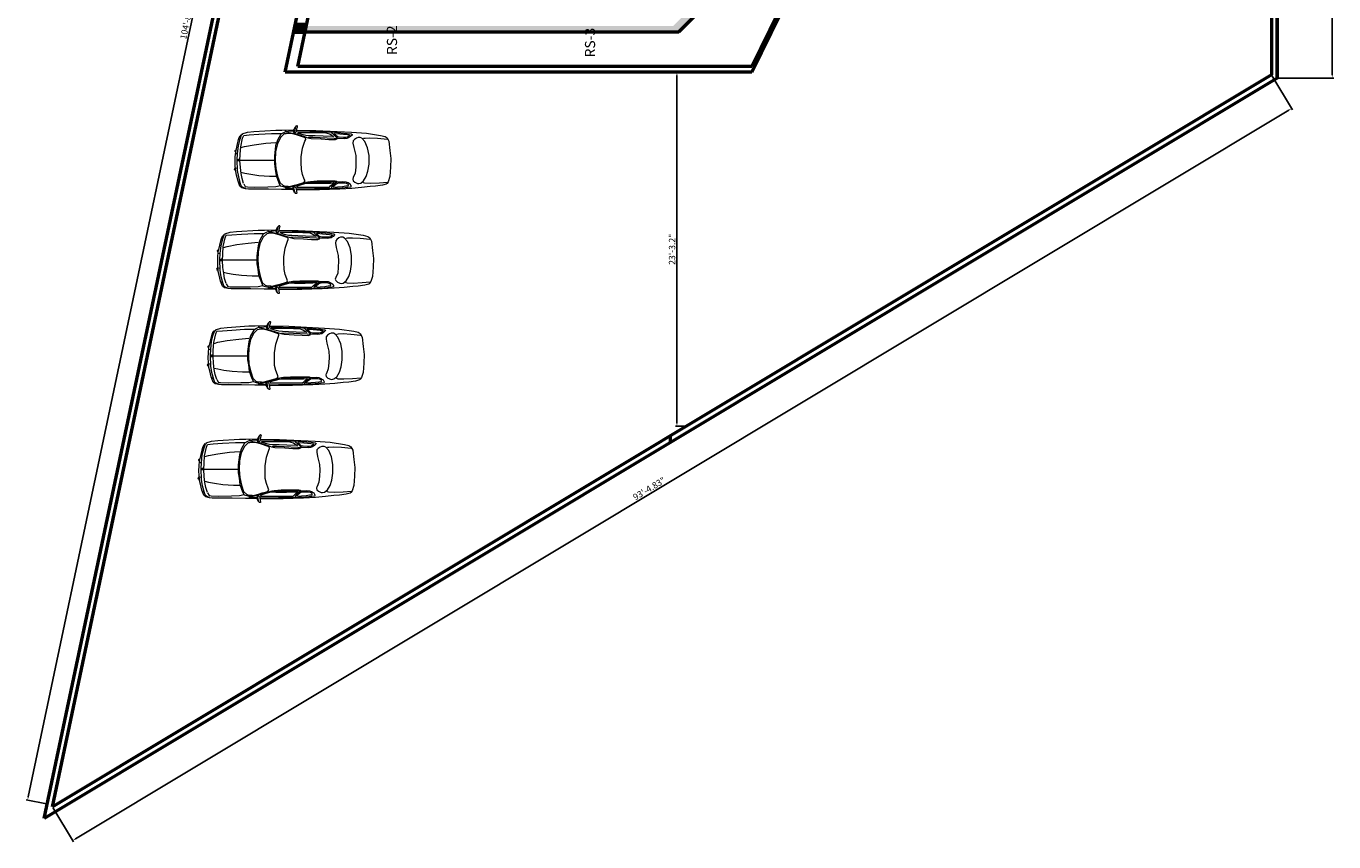
# Model space of a CAD drawing. Units: inches. Extents: x -2733 to 3435, y -338 to 1843.
# Tile 1 of 7: x -2733 to -1702, y -338 to 305. Entities that reach past the tile are written whole.
import ezdxf

# ---------------------------------------------------------------- set-up
doc = ezdxf.new("R2010")
doc.units = ezdxf.units.IN
doc.header["$PDMODE"] = 34
for name, color, linetype, lineweight in [('A-ANNO-DIMS', 2, 'Continuous', 18), ('A-ANNO-TEXT', 7, 'Continuous', 18), ('A-COLS', 1, 'Continuous', 35), ('A-WALL', 7, 'Continuous', 50), ('A-WALL-PATT', 8, 'Continuous', 13), ('C-PRKG', 8, 'Continuous', 18)]:
    doc.layers.add(name, color=color, linetype=linetype, lineweight=lineweight)
doc.styles.get("Standard").update_dxf_attribs({"font": 'arial.ttf'})
doc.styles.add('YQ_DIM', font='SUPEROS.SHX', dxfattribs={"width": 0.8, "bigfont": 'HZDX.SHX'})
doc.dimstyles.new('ISO-25', dxfattribs={"dimtxt": 5, "dimasz": 2.5, "dimexe": 1.25, "dimexo": 0.625, "dimtad": 1, "dimlunit": 3, "dimtxsty": 'Standard', "dimcen": 2.5, "dimadec": 0, "dimazin": 0, "dimtfac": 1, "dimtmove": 0, "dimatfit": 3, "dimfxl": 1, "dimarcsym": 0})

# ---------------------------------------------------------------- blocks, each defined once
blk = doc.blocks.new('A$C52303110')
for p, q in [((-1.969, 0.76), (-1.928, 0.839)), ((-1.928, 0.839), (-1.887, 0.875)), ((-1.928, 0.738), (-1.881, 0.868)), ((-1.881, 0.868), (-1.846, 0.889)), ((-1.863, 0.896), (-1.693, 0.951)), ((-1.852, 0.767), (-1.816, 0.853)), ((-1.816, 0.853), (-1.64, 0.868)), ((-1.693, 0.951), (-1.496, 0.973)), ((-1.64, 0.868), (-1.339, 0.889)), ((-1.496, 0.973), (-0.807, 1.016)), ((-1.339, 0.889), (-0.939, 0.911)), ((-0.939, 0.911), (-0.698, 0.911)), ((-0.807, 1.016), (-0.61, 1.016)), ((-0.647, 0.889), (-0.755, 0.7)), ((-0.698, 0.911), (-0.627, 0.911)), ((-0.539, 0.897), (-0.654, 0.79)), ((-0.56, 0.938), (-0.647, 0.889)), ((-0.61, 1.016), (-0.252, 1.027)), ((-0.499, 0.963), (-0.56, 0.938)), ((-0.479, 0.905), (-0.539, 0.897)), ((-0.517, 1.02), (-0.48, 0.966)), ((-0.404, 0.972), (-0.499, 0.963)), ((-0.48, 0.966), (-0.383, 0.946)), ((-0.371, 0.914), (-0.479, 0.905)), ((-0.256, 0.988), (-0.404, 0.972)), ((-0.383, 0.946), (-0.161, 0.897)), ((-0.263, 0.897), (-0.371, 0.914)), ((-0.115, 0.856), (-0.263, 0.897)), ((-0.237, 1.032), (-0.251, 1.001)), ((-0.251, 1.001), (-0.25, 0.98)), ((-0.25, 0.98), (-0.245, 0.957)), ((-0.245, 0.957), (-0.234, 0.947)), ((-0.198, 1.106), (-0.237, 1.032)), ((-0.234, 0.947), (-0.213, 0.938)), ((-0.206, 1.035), (-0.226, 0.944)), ((-0.213, 0.938), (-0.192, 0.936)), ((-0.185, 1.111), (-0.206, 1.035)), ((-0.184, 1.117), (-0.198, 1.106)), ((-0.192, 0.936), (-0.179, 0.942)), ((-0.168, 1.141), (-0.185, 1.111)), ((-0.179, 0.942), (-0.167, 0.957)), ((-0.162, 1.148), (-0.168, 1.141)), ((-0.167, 0.957), (-0.154, 0.98)), ((-0.142, 1.15), (-0.162, 1.148)), ((-0.161, 0.897), (0.098, 0.813)), ((-0.154, 0.98), (-0.148, 1.013)), ((-0.148, 1.013), (-0.144, 1.04)), ((-0.145, 0.991), (0.272, 0.981)), ((-0.144, 1.04), (-0.137, 1.07)), ((-0.144, 1.016), (0.455, 1.005)), ((-0.13, 1.15), (-0.142, 1.15)), ((-0.137, 1.07), (-0.123, 1.109)), ((-0.123, 1.145), (-0.13, 1.15)), ((-0.117, 1.134), (-0.123, 1.145)), ((-0.123, 1.109), (-0.117, 1.134)), ((-0.119, 0.926), (-0.109, 0.937)), ((0.017, 0.88), (-0.119, 0.926)), ((0.101, 0.782), (-0.115, 0.856)), ((-0.109, 0.937), (-0.091, 0.944)), ((-0.091, 0.944), (0.26, 0.948)), ((0.143, 0.85), (0.017, 0.88)), ((0.257, 0.843), (0.143, 0.85)), ((0.441, 0.835), (0.257, 0.843)), ((0.26, 0.948), (0.598, 0.941)), ((0.272, 0.981), (0.721, 0.966)), ((0.69, 0.824), (0.441, 0.835)), ((0.455, 1.005), (1.583, 0.951)), ((0.598, 0.941), (0.777, 0.937)), ((0.721, 0.966), (1.045, 0.951)), ((0.777, 0.937), (0.817, 0.926)), ((0.817, 0.926), (0.897, 0.896)), ((0.897, 0.896), (1.001, 0.832)), ((0.956, 0.951), (0.952, 0.971)), ((0.96, 0.926), (0.956, 0.951)), ((1.016, 0.877), (0.96, 0.926)), ((1.001, 0.832), (1.022, 0.813)), ((1.105, 0.798), (1.016, 0.877)), ((1.038, 0.912), (1.054, 0.916)), ((1.043, 0.899), (1.038, 0.912)), ((1.082, 0.858), (1.043, 0.899)), ((1.045, 0.951), (1.453, 0.917)), ((1.054, 0.916), (1.221, 0.903)), ((1.141, 0.807), (1.082, 0.858)), ((1.221, 0.903), (1.447, 0.882)), ((1.447, 0.882), (1.506, 0.871)), ((1.453, 0.917), (1.579, 0.897)), ((1.508, 0.83), (1.464, 0.796)), ((1.506, 0.871), (1.524, 0.86)), ((1.527, 0.847), (1.508, 0.83)), ((1.524, 0.86), (1.527, 0.847)), ((1.603, 0.862), (1.555, 0.818)), ((1.579, 0.897), (1.611, 0.882)), ((1.583, 0.951), (2.058, 0.918)), ((1.611, 0.882), (1.603, 0.862)), ((2.058, 0.918), (2.505, 0.852)), ((2.505, 0.852), (2.648, 0.819)), ((-2.069, 0.322), (-2.022, 0.537)), ((-2.022, 0.537), (-1.969, 0.76)), ((-2.01, 0.285), (-1.981, 0.523)), ((-1.981, 0.523), (-1.928, 0.738)), ((-1.975, 0.702), (-1.934, 0.738)), ((-1.928, 0.257), (-1.91, 0.494)), ((-1.91, 0.494), (-1.852, 0.767)), ((-1.904, 0.465), (-1.787, 0.501)), ((-1.787, 0.501), (-1.487, 0.559)), ((-1.487, 0.559), (-1.122, 0.602)), ((-1.122, 0.602), (-0.804, 0.631)), ((-0.809, 0.518), (-0.849, 0.206)), ((-0.755, 0.7), (-0.809, 0.518)), ((-0.755, 0.585), (-0.809, 0.329)), ((-0.654, 0.79), (-0.755, 0.585)), ((0, 0.173), (0.04, 0.445)), ((0.04, 0.445), (0.115, 0.667)), ((0.098, 0.813), (0.203, 0.778)), ((0.142, 0.757), (0.101, 0.782)), ((0.115, 0.667), (0.142, 0.724)), ((0.142, 0.724), (0.142, 0.757)), ((0.203, 0.778), (0.312, 0.754)), ((0.268, 0.783), (0.22, 0.783)), ((0.361, 0.788), (0.268, 0.783)), ((0.312, 0.754), (0.624, 0.739)), ((0.6, 0.778), (0.361, 0.788)), ((1.037, 0.759), (0.6, 0.778)), ((0.624, 0.739), (0.871, 0.724)), ((1.022, 0.813), (0.69, 0.824)), ((0.871, 0.724), (1.077, 0.719)), ((1.364, 0.748), (1.037, 0.759)), ((1.077, 0.719), (1.13, 0.739)), ((1.138, 0.763), (1.105, 0.798)), ((1.13, 0.739), (1.138, 0.763)), ((1.159, 0.801), (1.141, 0.807)), ((1.199, 0.794), (1.159, 0.801)), ((1.338, 0.788), (1.199, 0.794)), ((1.403, 0.79), (1.338, 0.788)), ((1.437, 0.759), (1.364, 0.748)), ((1.464, 0.796), (1.403, 0.79)), ((1.494, 0.773), (1.437, 0.759)), ((1.555, 0.818), (1.494, 0.773)), ((1.638, 0.675), (1.632, 0.604)), ((1.632, 0.604), (1.655, 0.471)), ((1.678, 0.724), (1.638, 0.675)), ((1.655, 0.471), (1.718, 0.217)), ((1.742, 0.767), (1.678, 0.724)), ((1.794, 0.788), (1.742, 0.767)), ((1.863, 0.788), (1.794, 0.788)), ((1.915, 0.76), (1.863, 0.788)), ((2.007, 0.661), (1.915, 0.76)), ((1.955, 0.738), (1.967, 0.76)), ((1.967, 0.76), (2.013, 0.767)), ((2.094, 0.457), (2.007, 0.661)), ((2.013, 0.767), (2.169, 0.774)), ((2.14, 0.217), (2.094, 0.457)), ((2.169, 0.774), (2.411, 0.76)), ((2.411, 0.76), (2.717, 0.731)), ((2.648, 0.819), (2.711, 0.776)), ((2.711, 0.776), (2.765, 0.666)), ((2.765, 0.666), (2.8, 0.371)), ((-2.087, 0.379), (-2.099, 0.364)), ((-2.099, 0.364), (-2.099, 0.35)), ((-2.099, 0.35), (-2.087, 0.343)), ((-2.064, 0.386), (-2.087, 0.379)), ((-2.087, 0.343), (-2.069, 0.336)), ((-2.087, 0.012), (-2.081, 0.17)), ((-2.081, -0.132), (-2.087, 0.012)), ((-2.081, 0.17), (-2.069, 0.322)), ((-2.057, 0.278), (-2.022, 0.285)), ((-2.022, 0.077), (-2.01, 0.285)), ((-2.01, -0.254), (-2.022, 0.077)), ((-1.981, 0.093), (-1.999, 0.079)), ((-1.999, 0.079), (-1.999, 0.064)), ((-1.999, 0.057), (-1.97, 0.057)), ((-1.963, 0.093), (-1.981, 0.093)), ((-1.97, 0.057), (-1.958, 0.057)), ((-1.958, 0.079), (-1.963, 0.093)), ((-1.958, 0.057), (-1.958, 0.079)), ((-1.934, 0.055), (-1.928, 0.257)), ((-1.922, -0.16), (-1.934, 0.055)), ((-1.926, 0.072), (-0.858, 0.072)), ((-0.849, 0.206), (-0.849, -0.049)), ((-0.809, 0.329), (-0.823, 0.058)), ((-0.823, 0.058), (-0.802, -0.19)), ((0, 0), (0, 0.173)), ((0.007, -0.23), (0, 0)), ((1.718, 0.217), (1.724, 0.033)), ((1.724, 0.033), (1.718, -0.15)), ((2.14, -0.058), (2.14, 0.217)), ((2.8, 0.371), (2.828, 0.12)), ((2.828, 0.12), (2.819, -0.153)), ((-2.11, -0.2), (-2.122, -0.221)), ((-2.122, -0.221), (-2.11, -0.236)), ((-2.093, -0.193), (-2.11, -0.2)), ((-2.11, -0.236), (-2.093, -0.25)), ((-2.069, -0.29), (-2.081, -0.132)), ((-2.04, -0.405), (-2.069, -0.29)), ((-2.064, -0.175), (-2.016, -0.182)), ((-1.993, -0.592), (-2.04, -0.405)), ((-1.975, -0.455), (-2.01, -0.254)), ((-1.898, -0.354), (-1.922, -0.16)), ((-1.903, -0.313), (-1.782, -0.341)), ((-1.869, -0.512), (-1.898, -0.354)), ((-1.782, -0.341), (-1.593, -0.376)), ((-1.593, -0.376), (-1.335, -0.411)), ((-1.335, -0.411), (-1.002, -0.432)), ((-0.849, -0.049), (-0.823, -0.214)), ((-0.823, -0.214), (-0.796, -0.412)), ((-0.802, -0.19), (-0.748, -0.436)), ((-0.796, -0.412), (-0.708, -0.642)), ((0.04, -0.387), (0.007, -0.23)), ((0.094, -0.527), (0.04, -0.387)), ((1.701, -0.34), (1.643, -0.481)), ((1.718, -0.15), (1.701, -0.34)), ((2.053, -0.446), (2.105, -0.277)), ((2.105, -0.277), (2.14, -0.058)), ((2.819, -0.153), (2.8, -0.448)), ((-1.934, -0.754), (-1.993, -0.592)), ((-1.916, -0.678), (-1.975, -0.455)), ((-1.975, -0.62), (-1.934, -0.642)), ((-1.872, -0.809), (-1.934, -0.754)), ((-1.881, -0.764), (-1.916, -0.678)), ((-1.816, -0.8), (-1.881, -0.764)), ((-1.755, -0.831), (-1.872, -0.809)), ((-1.822, -0.671), (-1.869, -0.512)), ((-1.816, -0.678), (-1.769, -0.764)), ((-1.752, -0.829), (-1.816, -0.8)), ((-1.769, -0.764), (-1.699, -0.771)), ((-1.699, -0.771), (-1.463, -0.778)), ((-1.463, -0.778), (-1.057, -0.771)), ((-1.057, -0.771), (-0.804, -0.764)), ((-1.002, -0.432), (-0.784, -0.432)), ((-0.804, -0.764), (-0.657, -0.735)), ((-0.748, -0.436), (-0.681, -0.634)), ((-0.708, -0.642), (-0.661, -0.741)), ((-0.681, -0.634), (-0.586, -0.724)), ((-0.661, -0.741), (-0.573, -0.766)), ((-0.586, -0.724), (-0.519, -0.749)), ((-0.573, -0.766), (-0.445, -0.799)), ((-0.519, -0.749), (-0.445, -0.749)), ((-0.503, -0.844), (-0.477, -0.811)), ((-0.477, -0.811), (-0.434, -0.788)), ((-0.445, -0.749), (-0.411, -0.749)), ((-0.445, -0.799), (-0.29, -0.823)), ((-0.434, -0.788), (-0.331, -0.774)), ((-0.398, -0.757), (-0.324, -0.749)), ((-0.331, -0.774), (-0.171, -0.732)), ((-0.324, -0.749), (-0.209, -0.716)), ((-0.267, -0.838), (-0.264, -0.809)), ((-0.264, -0.809), (-0.255, -0.789)), ((-0.255, -0.789), (-0.236, -0.778)), ((-0.236, -0.778), (-0.216, -0.773)), ((-0.232, -0.803), (-0.233, -0.779)), ((-0.221, -0.857), (-0.232, -0.803)), ((-0.216, -0.773), (-0.2, -0.775)), ((-0.209, -0.716), (-0.088, -0.683)), ((-0.2, -0.775), (-0.184, -0.792)), ((-0.184, -0.792), (-0.171, -0.809)), ((-0.171, -0.732), (-0.002, -0.68)), ((-0.171, -0.809), (-0.164, -0.829)), ((-0.132, -0.75), (-0.148, -0.778)), ((-0.148, -0.778), (-0.132, -0.783)), ((0.028, -0.704), (-0.132, -0.75)), ((-0.132, -0.783), (-0.067, -0.783)), ((-0.088, -0.683), (0.054, -0.642)), ((-0.067, -0.783), (0.147, -0.783)), ((-0.002, -0.68), (0.109, -0.643)), ((0.143, -0.671), (0.028, -0.704)), ((0.054, -0.642), (0.101, -0.617)), ((0.121, -0.585), (0.094, -0.527)), ((0.101, -0.617), (0.121, -0.585)), ((0.109, -0.643), (0.178, -0.62)), ((0.216, -0.662), (0.143, -0.671)), ((0.147, -0.783), (0.529, -0.783)), ((0.178, -0.62), (0.288, -0.601)), ((0.266, -0.629), (0.212, -0.624)), ((0.342, -0.666), (0.216, -0.662)), ((0.346, -0.634), (0.266, -0.629)), ((0.288, -0.601), (0.506, -0.587)), ((0.503, -0.671), (0.342, -0.666)), ((0.518, -0.634), (0.346, -0.634)), ((0.671, -0.666), (0.503, -0.671)), ((0.506, -0.587), (0.881, -0.587)), ((0.682, -0.629), (0.518, -0.634)), ((0.529, -0.783), (0.786, -0.783)), ((0.92, -0.662), (0.671, -0.666)), ((0.675, -0.83), (0.9, -0.825)), ((0.943, -0.624), (0.682, -0.629)), ((0.786, -0.783), (0.889, -0.783)), ((0.881, -0.587), (1.069, -0.587)), ((0.889, -0.783), (0.927, -0.746)), ((0.9, -0.825), (1.057, -0.816)), ((1.011, -0.652), (0.92, -0.662)), ((0.927, -0.746), (0.985, -0.69)), ((1.118, -0.615), (0.943, -0.624)), ((0.954, -0.788), (0.946, -0.82)), ((0.946, -0.82), (0.95, -0.839)), ((1, -0.722), (0.954, -0.788)), ((0.985, -0.69), (1.042, -0.657)), ((1.034, -0.741), (0.996, -0.783)), ((1.092, -0.648), (1, -0.722)), ((1.004, -0.783), (1.145, -0.774)), ((1.042, -0.657), (1.011, -0.652)), ((1.099, -0.69), (1.034, -0.741)), ((1.057, -0.816), (1.287, -0.802)), ((1.069, -0.587), (1.107, -0.592)), ((1.13, -0.629), (1.092, -0.648)), ((1.141, -0.662), (1.099, -0.69)), ((1.107, -0.592), (1.122, -0.606)), ((1.161, -0.62), (1.118, -0.615)), ((1.122, -0.606), (1.13, -0.629)), ((1.18, -0.657), (1.141, -0.662)), ((1.145, -0.774), (1.298, -0.76)), ((1.314, -0.615), (1.161, -0.62)), ((1.294, -0.652), (1.18, -0.657)), ((1.592, -0.82), (1.216, -0.842)), ((1.287, -0.802), (1.474, -0.783)), ((1.371, -0.652), (1.294, -0.652)), ((1.298, -0.76), (1.405, -0.746)), ((1.413, -0.62), (1.314, -0.615)), ((1.432, -0.666), (1.371, -0.652)), ((1.405, -0.746), (1.474, -0.741)), ((1.478, -0.648), (1.413, -0.62)), ((1.489, -0.704), (1.432, -0.666)), ((1.474, -0.741), (1.489, -0.727)), ((1.474, -0.783), (1.574, -0.769)), ((1.547, -0.69), (1.478, -0.648)), ((1.489, -0.727), (1.489, -0.704)), ((1.574, -0.732), (1.547, -0.69)), ((1.577, -0.76), (1.574, -0.732)), ((1.574, -0.769), (1.577, -0.76)), ((1.905, -0.798), (1.592, -0.82)), ((1.638, -0.481), (1.626, -0.531)), ((1.626, -0.531), (1.638, -0.58)), ((1.638, -0.58), (1.69, -0.629)), ((1.69, -0.629), (1.771, -0.664)), ((1.771, -0.664), (1.817, -0.671)), ((1.817, -0.671), (1.875, -0.657)), ((1.875, -0.657), (1.967, -0.587)), ((2.174, -0.766), (1.905, -0.798)), ((1.938, -0.615), (1.955, -0.636)), ((1.955, -0.636), (2.001, -0.65)), ((1.967, -0.587), (2.053, -0.446)), ((2.001, -0.65), (2.186, -0.657)), ((2.344, -0.754), (2.174, -0.766)), ((2.186, -0.657), (2.469, -0.643)), ((2.559, -0.722), (2.344, -0.754)), ((2.469, -0.643), (2.723, -0.622)), ((2.684, -0.689), (2.559, -0.722)), ((2.711, -0.667), (2.684, -0.689)), ((2.747, -0.612), (2.711, -0.667)), ((2.8, -0.448), (2.747, -0.612)), ((-1.666, -0.842), (-1.755, -0.831)), ((-1.55, -0.842), (-1.666, -0.842)), ((-1.039, -0.842), (-1.55, -0.842)), ((-0.619, -0.853), (-1.039, -0.842)), ((-0.279, -0.853), (-0.619, -0.853)), ((-0.254, -0.869), (-0.267, -0.838)), ((-0.233, -0.91), (-0.254, -0.869)), ((-0.217, -0.944), (-0.233, -0.91)), ((-0.205, -0.935), (-0.221, -0.857)), ((-0.2, -0.956), (-0.217, -0.944)), ((-0.196, -0.961), (-0.205, -0.935)), ((-0.192, -0.972), (-0.196, -0.961)), ((-0.178, -0.984), (-0.192, -0.972)), ((-0.166, -0.986), (-0.178, -0.984)), ((-0.152, -0.987), (-0.166, -0.986)), ((-0.164, -0.829), (-0.161, -0.849)), ((-0.161, -0.849), (-0.152, -0.906)), ((-0.155, -0.839), (0.124, -0.835)), ((-0.01, -0.864), (-0.153, -0.864)), ((-0.152, -0.906), (-0.143, -0.972)), ((-0.146, -0.982), (-0.152, -0.987)), ((-0.143, -0.972), (-0.146, -0.982)), ((0.572, -0.864), (-0.01, -0.864)), ((0.124, -0.835), (0.419, -0.83)), ((0.419, -0.83), (0.675, -0.83)), ((1.216, -0.842), (0.572, -0.864))]:
    blk.add_line(p, q)
blk = doc.blocks.new('*D5')
at = {"layer": 'A-ANNO-DIMS', "color": 0, "lineweight": -2, "transparency": 16777216}
for p, q in [((-2473, 922.1), (-2730.9, -302.7)), ((-2457.7, 921.4), (-2473.7, 924.8)), ((-2716.6, -308.3), (-2732.6, -304.9))]:
    blk.add_line(p, q, dxfattribs=at)
at = {"layer": 'A-ANNO-DIMS', "color": 0, "lineweight": 20, "transparency": 16777216}
for points in [[(-2473.4, 922.2), (-2472.6, 922), (-2472.5, 924.6)], [(-2731.3, -302.6), (-2730.5, -302.8), (-2731.4, -305.2)]]:
    blk.add_solid(points, dxfattribs=at)
at = {"layer": 'Defpoints', "color": 0, "lineweight": 20, "transparency": 16777216}
for p in [(-2457, 921.3), (-2731.4, -305.2), (-2715.9, -308.4)]:
    blk.add_point(p, dxfattribs=at)
at = {"layer": 'A-ANNO-DIMS', "color": 0, "transparency": 16777216, "insert": (-2605, 310.4), "char_height": 5, "attachment_point": 5, "rotation": 78.1108}
blk.add_mtext('104\'-8.67"', dxfattribs=at)
blk = doc.blocks.new('*D6')
at = {"layer": 'A-ANNO-DIMS', "color": 0, "lineweight": -2, "transparency": 16777216}
for p, q in [((-1745.9, 1560.1), (-1701.9, 1560.1)), ((-1703.2, 1557.6), (-1703.2, 266.6)), ((-1745.9, 264.1), (-1701.9, 264.1))]:
    blk.add_line(p, q, dxfattribs=at)
at = {"layer": 'A-ANNO-DIMS', "color": 0, "lineweight": 20, "transparency": 16777216}
for points in [[(-1703.6, 1557.6), (-1702.8, 1557.6), (-1703.2, 1560.1)], [(-1703.6, 266.6), (-1702.8, 266.6), (-1703.2, 264.1)]]:
    blk.add_solid(points, dxfattribs=at)
at = {"layer": 'Defpoints', "color": 0, "lineweight": 20, "transparency": 16777216}
for p in [(-1746.6, 1560.1), (-1746.6, 264.1), (-1703.2, 264.1)]:
    blk.add_point(p, dxfattribs=at)
at = {"layer": 'A-ANNO-DIMS', "color": 0, "transparency": 16777216, "insert": (-1706.4, 912.1), "char_height": 5, "attachment_point": 5, "rotation": 90}
blk.add_mtext("108'", dxfattribs=at)
blk = doc.blocks.new('*D7')
at = {"layer": 'A-ANNO-DIMS', "color": 0, "lineweight": -2, "transparency": 16777216}
for p, q in [((-1750.7, 266.1), (-1734.5, 239.1)), ((-1737.3, 238.9), (-2693.7, -335.8)), ((-2711.5, -311.1), (-2695.2, -338.2))]:
    blk.add_line(p, q, dxfattribs=at)
at = {"layer": 'A-ANNO-DIMS', "color": 0, "lineweight": 20, "transparency": 16777216}
for points in [[(-1737.5, 239.2), (-1737.1, 238.5), (-1735.1, 240.2)], [(-2694, -335.4), (-2693.5, -336.2), (-2695.9, -337.1)]]:
    blk.add_solid(points, dxfattribs=at)
at = {"layer": 'Defpoints', "color": 0, "lineweight": 20, "transparency": 16777216}
for p in [(-1751.1, 266.7), (-2711.8, -310.6), (-2695.9, -337.1)]:
    blk.add_point(p, dxfattribs=at)
at = {"layer": 'A-ANNO-DIMS', "color": 0, "transparency": 16777216, "insert": (-2241.2, -60.2), "char_height": 5, "attachment_point": 5, "rotation": 31}
blk.add_mtext('93\'-4.83"', dxfattribs=at)
blk = doc.blocks.new('*D19')
at = {"layer": 'A-ANNO-DIMS', "color": 0, "lineweight": -2, "transparency": 16777216}
for p, q in [((-2213.5, 268.7), (-2220.9, 268.7)), ((-2219.7, 266.2), (-2219.7, -8)), ((-2213, -10.5), (-2220.9, -10.5))]:
    blk.add_line(p, q, dxfattribs=at)
at = {"layer": 'A-ANNO-DIMS', "color": 0, "lineweight": 20, "transparency": 16777216}
for points in [[(-2220.1, 266.2), (-2219.3, 266.2), (-2219.7, 268.7)], [(-2220.1, -8), (-2219.3, -8), (-2219.7, -10.5)]]:
    blk.add_solid(points, dxfattribs=at)
at = {"layer": 'Defpoints', "color": 0, "lineweight": 20, "transparency": 16777216}
for p in [(-2212.9, 268.7), (-2219.7, -10.5), (-2212.4, -10.5)]:
    blk.add_point(p, dxfattribs=at)
at = {"layer": 'A-ANNO-DIMS', "color": 0, "transparency": 16777216, "insert": (-2222.9, 129.1), "char_height": 5, "attachment_point": 5, "rotation": 90}
blk.add_mtext('23\'-3.2"', dxfattribs=at)
blk = doc.blocks.new('*D22')
at = {"layer": 'A-ANNO-DIMS', "color": 0, "lineweight": -2, "transparency": 16777216}
blk.add_arc((-2457, 921.3), 20.3, 94.064, 251.0467, dxfattribs=at)
at = {"layer": 'A-ANNO-DIMS', "color": 0, "lineweight": 20, "transparency": 16777216}
for points in [[(-2458.5, 942), (-2458.5, 941.1), (-2456, 941.6)], [(-2463.5, 902.5), (-2463.7, 901.7), (-2461.2, 901.5)]]:
    blk.add_solid(points, dxfattribs=at)
at = {"layer": 'Defpoints', "color": 0, "lineweight": 20, "transparency": 16777216}
for p in [(-2423.6, 1560.1), (-2473.5, 933.2), (-2457, 921.3), (-2457, 921.3), (-2718.3, -319.8)]:
    blk.add_point(p, dxfattribs=at)
at = {"layer": 'A-ANNO-DIMS', "color": 0, "transparency": 16777216, "insert": (-2480.3, 924.3), "char_height": 5, "attachment_point": 5, "rotation": 82.5554}
blk.add_mtext('171°', dxfattribs=at)

msp = doc.modelspace()

# ---------------------------------------------------------------- hatches: boundary and pattern name
at = {"layer": 'A-COLS'}
h = msp.add_hatch(color=256, dxfattribs=at)
h.dxf.hatch_style = 1
h.paths.add_polyline_path([(-2512.158, 307.862), (-2521.158, 307.862), (-2521.158, 298.862), (-2512.158, 298.862)])
at = {"layer": 'A-WALL-PATT'}
h = msp.add_hatch(color=256, dxfattribs=at)
h.dxf.hatch_style = 1
h.paths.add_polyline_path([(-2182.126, 776.08), (-2186.626, 776.08), (-2186.626, 641.08), (-2182.126, 641.08)])
h.paths.add_polyline_path([(-2182.126, 932.085), (-2186.626, 932.085), (-2186.626, 792.58), (-2182.126, 792.58)])
h.paths.add_polyline_path([(-2182.126, 624.58), (-2186.626, 624.58), (-2186.626, 485.101), (-2182.126, 485.101)])
h.paths.add_polyline_path([(-2182.126, 468.606), (-2186.626, 468.606), (-2186.626, 341.08), (-2222.626, 305.08), (-2511.726, 305.08), (-2512.673, 300.58), (-2218.126, 300.58), (-2182.126, 336.58)])
h.paths.add_polyline_path([(-2182.126, 1088.154), (-2186.626, 1088.154), (-2186.626, 948.58), (-2182.126, 948.582)])
h.paths.add_polyline_path([(-2182.126, 1243.861), (-2186.626, 1243.861), (-2186.626, 1104.649), (-2182.126, 1104.649)])
h.paths.add_polyline_path([(-2182.126, 1340.024), (-2186.626, 1340.024), (-2186.626, 1260.356), (-2182.126, 1260.356)])
h.paths.add_polyline_path([(-2182.126, 1508.58), (-2186.626, 1508.58), (-2186.626, 1356.519), (-2182.126, 1356.519)])

# ---------------------------------------------------------------- linework, layer by layer
at = {"layer": 'A-WALL'}
for p, q in [((-1746.569, 1560.127), (-1746.569, 264.127)), ((-1751.069, 1555.627), (-1751.069, 266.673)), ((-2718.342, -319.774), (-2457.047, 921.314)), ((-2711.812, -310.6), (-2452.644, 920.386)), ((-2528.543, 268.651), (-2392.898, 912.931)), ((-2518.444, 273.153), (-2383.91, 912.46)), ((-1746.569, 264.127), (-1746.569, 729.127)), ((-2160.689, 273.202), (-2085.203, 428.08)), ((-2160.689, 268.702), (-2082.673, 428.08)), ((-2218.126, 300.58), (-2182.126, 336.58)), ((-2512.673, 300.58), (-2218.126, 300.58)), ((-2518.444, 268.653), (-2528.543, 268.651)), ((-1746.569, 264.127), (-2718.342, -319.774)), ((-1751.069, 266.673), (-2711.812, -310.6)), ((-2224.683, -23.153), (-2224.683, -17.903))]:
    msp.add_line(p, q, dxfattribs=at)
for points in [[(-2160.689, 273.202), (-2265.093, 273.202), (-2518.444, 273.153)], [(-2160.689, 268.702), (-2265.093, 268.702), (-2518.444, 268.653)]]:
    msp.add_lwpolyline(points, dxfattribs=at)

# ---------------------------------------------------------------- block references
at = {"layer": 'C-PRKG', "xscale": 24.97117926718032, "yscale": 24.97117926718032, "zscale": 24.97117926718032}
for p in [(-2515.773, 197.643), (-2529.533, 118.867), (-2536.938, 43.258), (-2544.286, -46.016)]:
    msp.add_blockref('A$C52303110', p, dxfattribs=at)

# ---------------------------------------------------------------- texts
at = {"layer": 'A-ANNO-TEXT', "char_height": 8, "attachment_point": 1, "rotation": 90, "style": 'YQ_DIM'}
for s, insert in [('{\\fSwis721 BlkCn BT|b0|i0|c0|p34;RS-2}', (-2448.274, 282.323)), ('{\\fSwis721 BlkCn BT|b0|i0|c0|p34;RS-3}', (-2292.166, 280.41))]:
    msp.add_mtext_dynamic_manual_height_columns(s, width=14.9584, gutter_width=12.5, heights=[0], dxfattribs=dict(at, insert=insert))

# ---------------------------------------------------------------- dimensions: what is measured, and where the dimension line sits
at = {"layer": 'A-ANNO-DIMS'}
dim = msp.add_angular_dim_2l(base=(-2473.47, 933.229), line1=((-2718.342, -319.774), (-2457.047, 921.314)), line2=((-2457.047, 921.314), (-2423.568, 1560.127)), dimstyle='ISO-25', override={"dimclrd": 0, "dimclre": 0, "dimclrt": 0}, dxfattribs=at)
dim.commit()
dim.dimension.update_dxf_attribs({"geometry": '*D22', "text_midpoint": (-2480.275, 924.349)})
for base, p1, p2, picture, middle in [((-1703.179, 264.127), (-1746.569, 1560.127), (-1746.569, 264.127), '*D6', (-1706.357, 912.127)), ((-2219.6727, -10.5026), (-2212.8907, 268.7018), (-2212.3658, -10.5026), '*D19', (-2222.8523, 129.0996))]:
    dim = msp.add_linear_dim(base=base, p1=p1, p2=p2, angle=90, dimstyle='ISO-25', override={"dimclrd": 0, "dimclre": 0, "dimclrt": 0}, dxfattribs=at)
    dim.commit()
    dim.dimension.update_dxf_attribs({"geometry": picture, "text_midpoint": middle})
dim = msp.add_aligned_dim(p1=(-2457.047, 921.314), p2=(-2715.948, -308.402), distance=-15.77, dimstyle='ISO-25', override={"dimclrd": 0, "dimclre": 0, "dimclrt": 0}, dxfattribs=at)
dim.commit()
dim.dimension.update_dxf_attribs({"geometry": '*D5', "text_midpoint": (-2605.039, 310.359)})
dim = msp.add_linear_dim(base=(-2695.89245, -337.09439), p1=(-1751.06875, 266.67263), p2=(-2711.81185, -310.60006), angle=211, dimstyle='ISO-25', override={"dimclrd": 0, "dimclre": 0, "dimclrt": 0}, dxfattribs=at)
dim.commit()
dim.dimension.update_dxf_attribs({"geometry": '*D7', "text_midpoint": (-2239.59926, -62.92578), "dimtype": 161})

doc.saveas('drawing.dxf')
